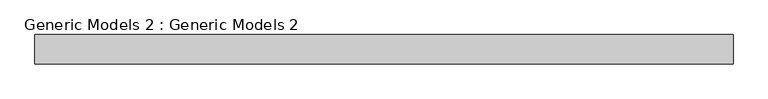
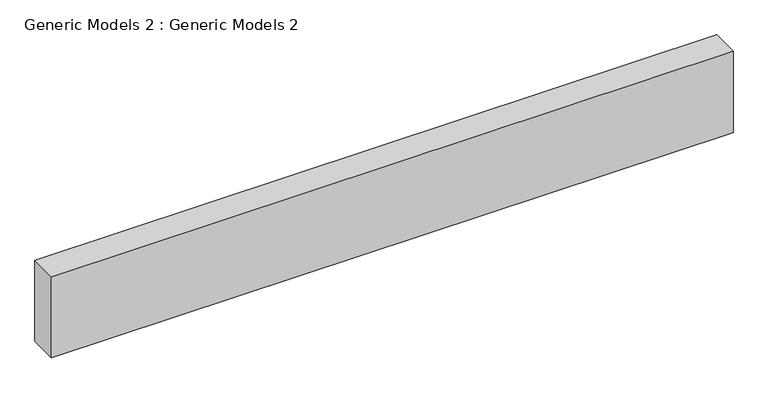
"""IFC4 building model written with IfcOpenShell, lengths in millimetres: proxy geometry, Generic Models 2 : Generic Models 2."""

from ifc_helpers import new_model, si_unit, frame, origin, place, context, project, spatial, polyline, outline, extrude, source, transform, mapped, element, save


def generic_models_2_generic_models_2_cf9e9294(model_context):
    return source(origin(), model_context, "Body", "SweptSolid", [
        extrude(outline(polyline([(-12049.6586008, -7754.7844117), (-4797.9586008, -7754.7844117), (-4797.9586008, -8059.5844117), (-12049.6586008, -8059.5844117), (-12049.6586008, -7754.7844117)])), frame((0.0, 0.0, 6400.8), z_axis=(0.0, 0.0, 1.0), x_axis=(1.0, 0.0, 0.0)), (0.0, 0.0, 1.0), 914.4),
    ])


if __name__ == "__main__":
    model = new_model("IFC4")
    model_context = context("Model", 3, world=origin())
    ifc_project = project(units=[si_unit("LENGTHUNIT", "METRE", prefix="MILLI")], contexts=[model_context])
    site = spatial("IfcSite", under=ifc_project)
    building = spatial("IfcBuilding", under=site)
    placement = place(None, origin())
    generic_models_2_generic_models_2_shape = generic_models_2_generic_models_2_cf9e9294(model_context)
    element("IfcBuildingElementProxy", 1, Name="Generic Models 2 : Generic Models 2", ObjectType="Generic Models 2 : Generic Models 2", at=placement, inside=building, context=model_context, shape_type="MappedRepresentation", body=[
        mapped(generic_models_2_generic_models_2_shape, transform((0.0, 0.0, 0.0), x_axis=(1.0, 0.0, 0.0), y_axis=(0.0, 1.0, 0.0), z_axis=(0.0, 0.0, 1.0))),
    ])
    save(model, "model.ifc")

# Revit data of these elements
# Element 1 (IfcBuildingElementProxy, "Generic Models 2 : Generic Models 2")
#   Materials on its faces: "ESPRESSO"
# Materials
#   "ESPRESSO": class "Generic", colour RGB 120 120 120, transparency 0, Cost = 0
